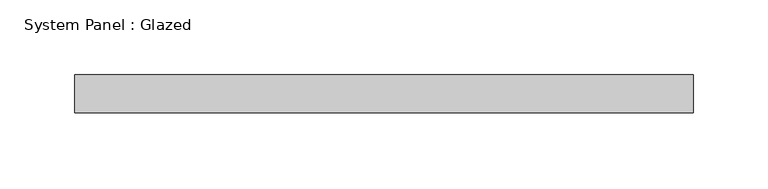
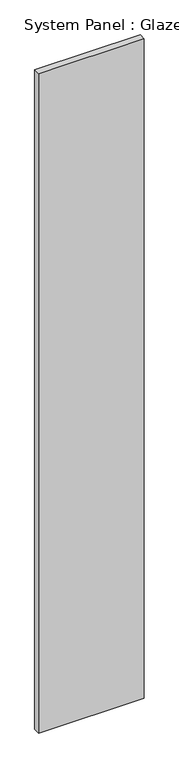
"""IFC4 building model written with IfcOpenShell, lengths in millimetres: plate geometry, System Panel : Glazed."""

from ifc_helpers import new_model, si_unit, origin, origin_with_axes, place, context, project, spatial, polyline, outline, extrude, source, transform, mapped, element, save


def system_panel_glazed_213fa7e9(model_context):
    return source(origin(), model_context, "Body", "SweptSolid", [
        extrude(outline(polyline([(206.375, 19.05), (-206.375, 19.05), (-206.375, 44.45), (206.375, 44.45), (206.375, 19.05)])), origin_with_axes(), (0.0, 0.0, 1.0), 2719.788773),
    ])


if __name__ == "__main__":
    model = new_model("IFC4")
    model_context = context("Model", 3, world=origin())
    ifc_project = project(units=[si_unit("LENGTHUNIT", "METRE", prefix="MILLI")], contexts=[model_context])
    site = spatial("IfcSite", under=ifc_project)
    building = spatial("IfcBuilding", under=site)
    placement = place(None, origin())
    system_panel_glazed_shape = system_panel_glazed_213fa7e9(model_context)
    element("IfcPlate", 1, ObjectType="System Panel : Glazed", at=placement, inside=building, context=model_context, shape_type="MappedRepresentation", body=[
        mapped(system_panel_glazed_shape, transform((0.0, 0.0, 0.0), x_axis=(1.0, 0.0, 0.0), y_axis=(0.0, 1.0, 0.0), z_axis=(0.0, 0.0, 1.0))),
    ])
    save(model, "model.ifc")

# Revit data of these elements
# Type "System Panel : Glazed"
#   Construction Type Id = "GSP4R"
#   Analytic Construction = "1/8 in Pilkington single glazing"
#   Visual Light Transmittance = 0.9
#   Solar Heat Gain Coefficient = 0.86
#   Heat Transfer Coefficient (U) = 1.18115 BTU/(h·ft²·°F)
# Element 1 (IfcPlate, "System Panel : Glazed")
#   Materials on its faces: "Glass"
# Materials
#   "Glass": class "Glass", colour RGB 0 128 192, transparency 0.75, Description = "Soda Lime Glass", Cost = 0
